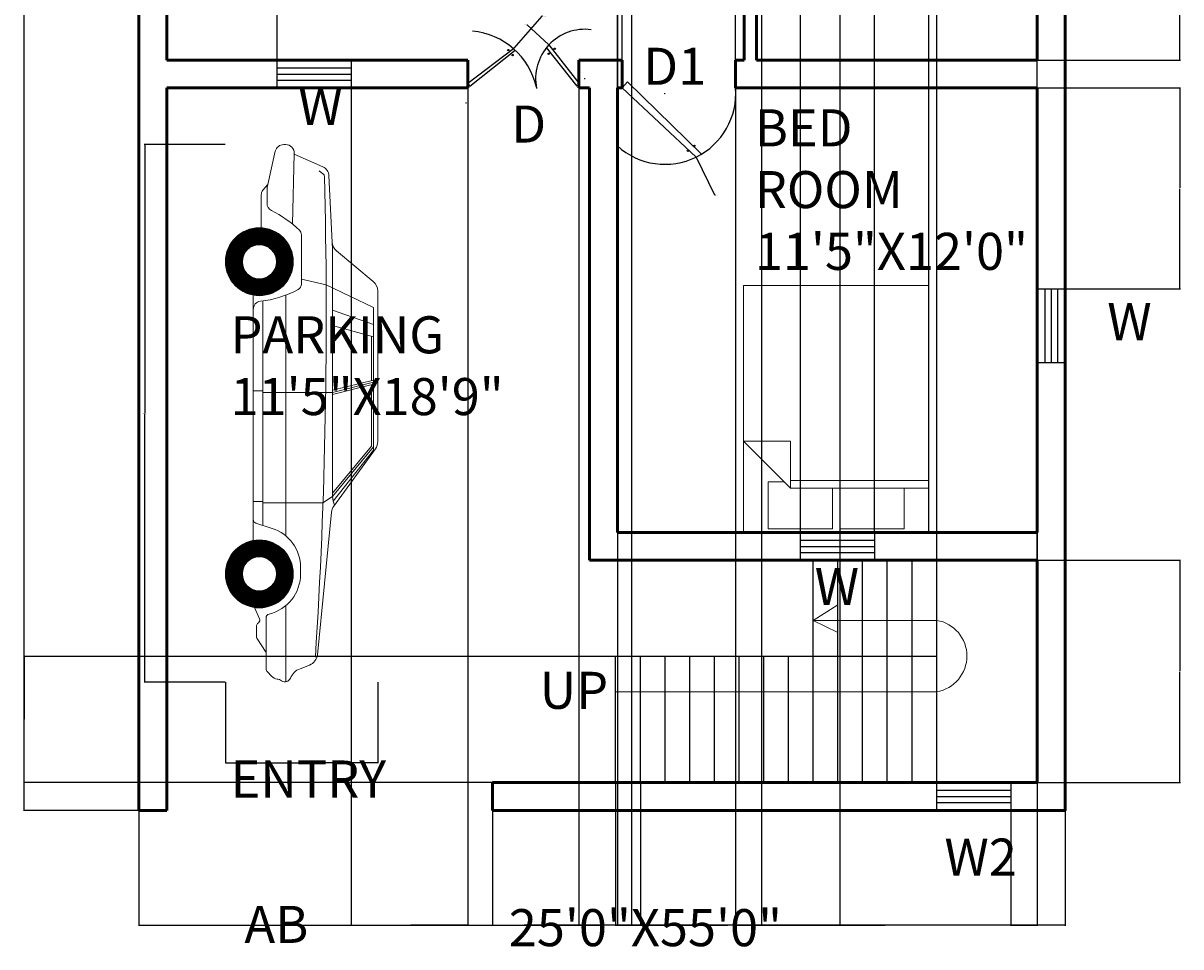
# Model space of a CAD drawing. Units: inches. Extents: x -15 to 361, y -684 to 58.
# Tile 1 of 3: x -15 to 360, y -684 to -385. Entities that reach past the tile are written whole.
import ezdxf

# ---------------------------------------------------------------- set-up
doc = ezdxf.new("R2010")
doc.units = ezdxf.units.IN
doc.header["$MEASUREMENT"] = 0
for name, color, linetype, lineweight in [('A-ANNO-DIMS', 2, 'Continuous', 18), ('A-ANNO-SYMB', 2, 'Continuous', 18), ('A-ANNO-TEXT', 7, 'Continuous', 18), ('A-AREA-IDEN', 7, 'Continuous', 25), ('A-DOOR', 3, 'Continuous', 25), ('A-EQPM-VEHC', 9, 'Continuous', 18), ('A-FLOR-STRS', 7, 'Continuous', 25), ('A-FURN', 8, 'Continuous', 18), ('A-GLAZ', 4, 'Continuous', 25), ('A-WALL', 7, 'Continuous', 50)]:
    doc.layers.add(name, color=color, linetype=linetype, lineweight=lineweight)
doc.styles.get("Standard").update_dxf_attribs({"font": 'arial.ttf'})
doc.dimstyles.get("Standard").update_dxf_attribs({"dimtxt": 0.18, "dimasz": 0.18, "dimexe": 0.18, "dimexo": 0.0625, "dimgap": 0.09, "dimtad": 0, "dimtih": 1, "dimtoh": 1, "dimdec": 4, "dimzin": 0, "dimdsep": 46, "dimtxsty": 'Standard', "dimcen": 0.09, "dimadec": 0, "dimazin": 0, "dimtfac": 1, "dimtdec": 4, "dimtofl": 0, "dimtmove": 0, "dimatfit": 3, "dimfxl": 1, "dimtolj": 1, "dimtzin": 0, "dimarcsym": 0})

# ---------------------------------------------------------------- blocks, each defined once
blk = doc.blocks.new('Bed - Queen')
for p, q in [((0, -80.00003), (0, 0)), ((0, 0), (59.99999, 0)), ((59.99999, 0), (59.99999, -80.00003)), ((7.99999, -1.2), (28.79998, -1.2)), ((7.99999, -14.4), (7.99999, -1.2)), ((28.79998, -1.2), (28.79998, -14.4)), ((31.19999, -1.2), (51.99999, -1.2)), ((31.19999, -14.4), (31.19999, -1.2)), ((51.99999, -1.2), (51.99999, -16.4)), ((0, -14.4), (44.8, -14.4)), ((59.99999, -29.6), (44.8, -14.4)), ((44.8, -14.4), (44.8, -29.6)), ((44.8, -16.8), (0, -16.8)), ((51.99999, -16.4), (46.79936, -16.4)), ((44.8, -29.6), (59.99999, -29.6)), ((59.99999, -80.00003), (0, -80.00003))]:
    blk.add_line(p, q)
blk = doc.blocks.new('Car - sedan  side')
for p, q in [((-77.81, 49.34), (-126.58, 49.34)), ((-139.53, 35.99), (-129.64, 47.91)), ((-128.57, 32.64), (-121.22, 48.02)), ((-74.7, 48.02), (-121.22, 48.02)), ((-120.32, 34.67), (-115.67, 48.02)), ((-115.4, 34.67), (-111.74, 48.02)), ((-97.55, 47.3), (-111.94, 47.3)), ((-94.41, 34.67), (-97.73, 48.02)), ((-93.72, 34.67), (-97.04, 48.02)), ((-93.03, 34.67), (-96.34, 48.02)), ((-76.26, 47.3), (-96.16, 47.3)), ((-61.08, 34.66), (-76.26, 47.3)), ((-60.02, 34.65), (-76.07, 48.02)), ((-56.87, 35.13), (-75.48, 48.59)), ((-58.54, 34.93), (-74.99, 48.02)), ((-140.23, 34.67), (-163.88, 33.56)), ((-62.28, 34.67), (-140.23, 34.67)), ((-93.72, 19.62), (-93.72, 34.67)), ((-62.28, 34.67), (-60.02, 34.65)), ((-60.02, 34.65), (-58.54, 34.93)), ((-57.97, 31.61), (-60.02, 34.65)), ((-57.21, 35.38), (-58.54, 34.93)), ((-54.93, 34.4), (-8.75, 29.8)), ((-170.93, 22.32), (-166.81, 31.56)), ((-164.57, 31.6), (-165.48, 30.35)), ((-130.39, 24.63), (-128.57, 32.64)), ((-57.97, 19.62), (-57.97, 31.61)), ((-4.21, 24.18), (-5.42, 27.27)), ((-128.78, 24.63), (-144.79, 24.63)), ((-36.97, 24.38), (-34.94, 24.38)), ((-174, 19.51), (-174, 18.91)), ((-148.26, 21.7), (-171.11, 22.33)), ((-47.2, 19.62), (-125.23, 19.62)), ((-93.72, 12.14), (-93.72, 19.62)), ((-57.97, 12.14), (-57.97, 19.62)), ((0, 19.62), (-24.7, 19.62)), ((-160.12, 13.48), (-171.81, 16.16)), ((-51.4, 9.89), (-49.69, 15.14)), ((-159.22, 12.14), (-161.08, 13.7)), ((-155.01, 13.48), (-160.12, 13.48)), ((-147.03, 11.6), (-157.73, 11.6)), ((-50.67, 12.14), (-123.32, 12.14)), ((-94.21, 9.03), (-94.21, 12.14)), ((-58.39, 9.03), (-58.39, 12.14)), ((-4.23, 13.19), (-20.72, 13.19)), ((-9.5, 13.19), (-14.1, 10.2)), ((-3.22, 13.59), (-1.77, 14.97)), ((-120.62, 9.03), (-125.23, 9.03)), ((-45.76, 9.03), (-120.62, 9.03)), ((-20.36, 11.06), (-24.06, 9.44)), ((-18.83, 10.42), (-19.11, 10.76)), ((-14.68, 10.03), (-18.01, 10.03))]:
    blk.add_line(p, q)
at = {"const_width": 5.49}
for points in [[(-127.8, 11, -1), (-144.3, 11, -1)], [(-26.69, 11, -1), (-43.19, 11, -1)]]:
    blk.add_lwpolyline(points, format="xyb", close=True, dxfattribs=at)
for centre, radius in [((-136.05, 11), 11), ((-34.94, 11), 11), ((-136.05, 11), 5.51), ((-34.94, 11), 5.51)]:
    blk.add_circle(centre, radius)
for centre, radius, start, end in [((-126.58, 45.38), 3.97, 90, 140.3029), ((-77.81, 45.38), 3.97, 54.135, 90), ((-142.58, 38.53), 3.97, 272.6827, 320.3029), ((-54.54, 38.35), 3.97, 234.135, 264.3123), ((-163.72, 30.18), 3.38, 92.6827, 155.9736), ((-163.62, 30.91), 1.17, 91.491, 143.9553), ((-118.51, -1702.12), 1734.79, 86.34698, 91.49105), ((-9.15, 25.82), 4, 21.3107, 84.3123), ((-118.09, -2.78), 38.85, 136.3964, 152.9097), ((-144.79, 22.64), 1.98, 90, 136.3964), ((-128.78, 22.64), 1.98, 28.1371, 90), ((-157.14, 7.48), 34.14, 6.5135, 28.1371), ((-36.97, 11), 13.38, 90, 161.9732), ((-34.94, 11), 13.38, 13.5864, 90), ((0.9, 26.18), 5.49, 201.3107, 247.7048), ((-171.18, 19.51), 2.82, 88.4193, 180), ((-171.18, 18.91), 2.82, 180, 257.0905), ((-1.92, 19.3), 1.94, 325.3744, 67.7048), ((-3.82, 17.12), 2.96, 313.7173, 352.3839), ((2.46, 16.28), 3.37, 145.3744, 172.3839), ((-157.73, 13.93), 2.32, 230.1291, 270), ((-155.01, 16.1), 2.62, 270, 332.9097), ((-120.62, 11.65), 2.62, 186.5135, 270), ((-20.72, 14.43), 1.24, 193.5864, 270), ((-4.23, 14.65), 1.46, 270, 313.7173), ((-52.58, 10.27), 1.24, 270, 341.9732), ((-19.93, 10.09), 1.06, 39.301, 113.7159), ((-18.01, 11.09), 1.06, 219.301, 270), ((-14.68, 11.09), 1.06, 270, 303.047)]:
    blk.add_arc(centre, radius, start, end)
blk = doc.blocks.new('WIN-24IN')
for p, q in [((0, 6.5), (24, 6.5)), ((0, 4.5), (24, 4.5)), ((0, 2.5), (24, 2.5))]:
    blk.add_line(p, q)
blk.add_lwpolyline([(0, 9), (24, 9), (24, 0), (0, 0)], close=True)
blk = doc.blocks.new('*D21')
at = {"layer": 'A-ANNO-DIMS', "color": 0, "lineweight": -2, "transparency": 16777216}
for p, q in [((50.87, -424.03), (24.63, -424.03)), ((24.81, -424.21), (24.81, -510.91)), ((24.81, -597.97), (24.81, -511.27)), ((50.87, -598.15), (24.63, -598.15))]:
    blk.add_line(p, q, dxfattribs=at)
at = {"layer": 'A-ANNO-DIMS', "color": 0, "transparency": 16777216}
for points in [[(24.78, -424.21), (24.84, -424.21), (24.81, -424.03)], [(24.78, -597.97), (24.84, -597.97), (24.81, -598.15)]]:
    blk.add_solid(points, dxfattribs=at)
at = {"layer": 'Defpoints', "color": 0, "transparency": 16777216}
for p in [(50.93, -424.03), (24.81, -598.15), (50.93, -598.15)]:
    blk.add_point(p, dxfattribs=at)
at = {"layer": 'A-ANNO-DIMS', "color": 0, "transparency": 16777216, "insert": (24.81, -511.09), "char_height": 0.18, "attachment_point": 5}
blk.add_mtext('\\A1;SEDAN 174', dxfattribs=at)
blk = doc.blocks.new('*D22')
at = {"layer": 'A-ANNO-DIMS', "color": 0, "lineweight": -2, "transparency": 16777216}
for p, q in [((50.93, -598.21), (50.93, -624.44)), ((100.28, -598.21), (100.28, -624.44)), ((51.11, -624.26), (75.38, -624.26)), ((100.1, -624.26), (75.83, -624.26))]:
    blk.add_line(p, q, dxfattribs=at)
at = {"layer": 'A-ANNO-DIMS', "color": 0, "transparency": 16777216}
for points in [[(51.11, -624.23), (51.11, -624.29), (50.93, -624.26)], [(100.1, -624.23), (100.1, -624.29), (100.28, -624.26)]]:
    blk.add_solid(points, dxfattribs=at)
at = {"layer": 'Defpoints', "color": 0, "transparency": 16777216}
for p in [(50.93, -598.15), (100.28, -598.15), (100.28, -624.26)]:
    blk.add_point(p, dxfattribs=at)
at = {"layer": 'A-ANNO-DIMS', "color": 0, "transparency": 16777216, "insert": (75.6, -624.26), "char_height": 0.18, "attachment_point": 5}
blk.add_mtext('\\A1;49', dxfattribs=at)
blk = doc.blocks.new('*D23')
at = {"layer": 'A-ANNO-DIMS', "color": 0, "lineweight": -2, "transparency": 16777216}
for p, q in [((22.93, -639.75), (22.93, -677.07)), ((322.93, -639.75), (322.93, -677.07)), ((23.11, -676.89), (172.64, -676.89)), ((322.75, -676.89), (173.22, -676.89))]:
    blk.add_line(p, q, dxfattribs=at)
at = {"layer": 'A-ANNO-DIMS', "color": 0, "transparency": 16777216}
for points in [[(23.11, -676.86), (23.11, -676.92), (22.93, -676.89)], [(322.75, -676.86), (322.75, -676.92), (322.93, -676.89)]]:
    blk.add_solid(points, dxfattribs=at)
at = {"layer": 'Defpoints', "color": 0, "transparency": 16777216}
for p in [(22.93, -639.69), (322.93, -639.69), (322.93, -676.89)]:
    blk.add_point(p, dxfattribs=at)
at = {"layer": 'A-ANNO-DIMS', "color": 0, "transparency": 16777216, "insert": (172.93, -676.89), "char_height": 0.18, "attachment_point": 5}
blk.add_mtext('\\A1;300', dxfattribs=at)
blk = doc.blocks.new('*D24')
at = {"layer": 'A-ANNO-DIMS', "color": 0, "lineweight": -2, "transparency": 16777216}
for p, q in [((22.87, 20.31), (-14.45, 20.31)), ((-14.27, 20.13), (-14.27, -309.51)), ((-14.27, -639.51), (-14.27, -309.87)), ((22.87, -639.69), (-14.45, -639.69))]:
    blk.add_line(p, q, dxfattribs=at)
at = {"layer": 'A-ANNO-DIMS', "color": 0, "transparency": 16777216}
for points in [[(-14.3, 20.13), (-14.24, 20.13), (-14.27, 20.31)], [(-14.3, -639.51), (-14.24, -639.51), (-14.27, -639.69)]]:
    blk.add_solid(points, dxfattribs=at)
at = {"layer": 'Defpoints', "color": 0, "transparency": 16777216}
for p in [(-14.27, 20.31), (22.93, 20.31), (22.93, -639.69)]:
    blk.add_point(p, dxfattribs=at)
at = {"layer": 'A-ANNO-DIMS', "color": 0, "transparency": 16777216, "insert": (-14.27, -309.69), "char_height": 0.18, "attachment_point": 5}
blk.add_mtext('\\A1;660', dxfattribs=at)
blk = doc.blocks.new('*D29')
at = {"layer": 'A-ANNO-DIMS', "color": 0, "lineweight": -2, "transparency": 16777216}
for p, q in [((313.99, -405.69), (360.31, -405.69)), ((360.13, -405.87), (360.13, -438.03)), ((360.13, -470.56), (360.13, -438.4)), ((313.99, -470.74), (360.31, -470.74))]:
    blk.add_line(p, q, dxfattribs=at)
at = {"layer": 'A-ANNO-DIMS', "color": 0, "transparency": 16777216}
for points in [[(360.1, -405.87), (360.16, -405.87), (360.13, -405.69)], [(360.1, -470.56), (360.16, -470.56), (360.13, -470.74)]]:
    blk.add_solid(points, dxfattribs=at)
at = {"layer": 'Defpoints', "color": 0, "transparency": 16777216}
for p in [(313.93, -405.69), (313.93, -470.74), (360.13, -470.74)]:
    blk.add_point(p, dxfattribs=at)
at = {"layer": 'A-ANNO-DIMS', "color": 0, "transparency": 16777216, "insert": (360.13, -438.22), "char_height": 0.18, "attachment_point": 5}
blk.add_mtext('\\A1;65.05', dxfattribs=at)
blk = doc.blocks.new('*D30')
at = {"layer": 'A-ANNO-DIMS', "color": 0, "lineweight": -2, "transparency": 16777216}
for p, q in [((305.35, -639.75), (305.35, -677.07)), ((322.93, -639.75), (322.93, -677.07)), ((305.53, -676.89), (313.68, -676.89)), ((322.75, -676.89), (314.6, -676.89))]:
    blk.add_line(p, q, dxfattribs=at)
at = {"layer": 'A-ANNO-DIMS', "color": 0, "transparency": 16777216}
for points in [[(305.53, -676.86), (305.53, -676.92), (305.35, -676.89)], [(322.75, -676.86), (322.75, -676.92), (322.93, -676.89)]]:
    blk.add_solid(points, dxfattribs=at)
at = {"layer": 'Defpoints', "color": 0, "transparency": 16777216}
for p in [(305.35, -639.69), (322.93, -639.69), (322.93, -676.89)]:
    blk.add_point(p, dxfattribs=at)
at = {"layer": 'A-ANNO-DIMS', "color": 0, "transparency": 16777216, "insert": (314.14, -676.89), "char_height": 0.18, "attachment_point": 5}
blk.add_mtext('\\A1;17.575', dxfattribs=at)
blk = doc.blocks.new('*D31')
at = {"layer": 'A-ANNO-DIMS', "color": 0, "lineweight": -2, "transparency": 16777216}
for p, q in [((177.93, -549.63), (177.93, 57.69)), ((178.11, 57.51), (207.18, 57.51)), ((237.04, 57.51), (207.97, 57.51)), ((237.22, -549.63), (237.22, 57.69))]:
    blk.add_line(p, q, dxfattribs=at)
at = {"layer": 'A-ANNO-DIMS', "color": 0, "transparency": 16777216}
for points in [[(178.11, 57.54), (178.11, 57.48), (177.93, 57.51)], [(237.04, 57.54), (237.04, 57.48), (237.22, 57.51)]]:
    blk.add_solid(points, dxfattribs=at)
at = {"layer": 'Defpoints', "color": 0, "transparency": 16777216}
for p in [(237.22, 57.51), (177.93, -549.69), (237.22, -549.69)]:
    blk.add_point(p, dxfattribs=at)
at = {"layer": 'A-ANNO-DIMS', "color": 0, "transparency": 16777216, "insert": (207.57, 57.51), "char_height": 0.18, "attachment_point": 5}
blk.add_mtext('\\A1;59.29', dxfattribs=at)
blk = doc.blocks.new('*D32')
at = {"layer": 'A-ANNO-DIMS', "color": 0, "lineweight": -2, "transparency": 16777216}
for p, q in [((31.93, -396.63), (31.93, 57.69)), ((32.11, 57.51), (49.42, 57.51)), ((67.52, 57.51), (50.21, 57.51)), ((67.7, -396.63), (67.7, 57.69))]:
    blk.add_line(p, q, dxfattribs=at)
at = {"layer": 'A-ANNO-DIMS', "color": 0, "transparency": 16777216}
for points in [[(32.11, 57.54), (32.11, 57.48), (31.93, 57.51)], [(67.52, 57.54), (67.52, 57.48), (67.7, 57.51)]]:
    blk.add_solid(points, dxfattribs=at)
at = {"layer": 'Defpoints', "color": 0, "transparency": 16777216}
for p in [(67.7, 57.51), (31.93, -396.69), (67.7, -396.69)]:
    blk.add_point(p, dxfattribs=at)
at = {"layer": 'A-ANNO-DIMS', "color": 0, "transparency": 16777216, "insert": (49.81, 57.51), "char_height": 0.18, "attachment_point": 5}
blk.add_mtext('\\A1;35.77', dxfattribs=at)
blk = doc.blocks.new('*D35')
at = {"layer": 'A-ANNO-DIMS', "color": 0, "lineweight": -2, "transparency": 16777216}
for p, q in [((137.49, -630.75), (137.49, -677.07)), ((177.35, -630.75), (177.35, -677.07)), ((137.67, -676.89), (157.03, -676.89)), ((177.17, -676.89), (157.82, -676.89))]:
    blk.add_line(p, q, dxfattribs=at)
at = {"layer": 'A-ANNO-DIMS', "color": 0, "transparency": 16777216}
for points in [[(137.67, -676.86), (137.67, -676.92), (137.49, -676.89)], [(177.17, -676.86), (177.17, -676.92), (177.35, -676.89)]]:
    blk.add_solid(points, dxfattribs=at)
at = {"layer": 'Defpoints', "color": 0, "transparency": 16777216}
for p in [(137.49, -630.69), (177.35, -630.69), (177.35, -676.89)]:
    blk.add_point(p, dxfattribs=at)
at = {"layer": 'A-ANNO-DIMS', "color": 0, "transparency": 16777216, "insert": (157.42, -676.89), "char_height": 0.18, "attachment_point": 5}
blk.add_mtext('\\A1;39.86', dxfattribs=at)
blk = doc.blocks.new('*D37')
at = {"layer": 'A-ANNO-DIMS', "color": 0, "lineweight": -2, "transparency": 16777216}
for p, q in [((182.53, -153.75), (182.53, -677.07)), ((224.64, -153.75), (224.64, -677.07)), ((182.71, -676.89), (203.21, -676.89)), ((224.46, -676.89), (203.97, -676.89))]:
    blk.add_line(p, q, dxfattribs=at)
at = {"layer": 'A-ANNO-DIMS', "color": 0, "transparency": 16777216}
for points in [[(182.71, -676.86), (182.71, -676.92), (182.53, -676.89)], [(224.46, -676.86), (224.46, -676.92), (224.64, -676.89)]]:
    blk.add_solid(points, dxfattribs=at)
at = {"layer": 'Defpoints', "color": 0, "transparency": 16777216}
for p in [(182.53, -153.69), (224.64, -153.69), (224.64, -676.89)]:
    blk.add_point(p, dxfattribs=at)
at = {"layer": 'A-ANNO-DIMS', "color": 0, "transparency": 16777216, "insert": (203.59, -676.89), "char_height": 0.18, "attachment_point": 5}
blk.add_mtext('\\A1;42.11', dxfattribs=at)
blk = doc.blocks.new('*D40')
at = {"layer": 'A-ANNO-DIMS', "color": 0, "lineweight": -2, "transparency": 16777216}
for p, q in [((91.7, -405.75), (91.7, -677.07)), ((129.45, -405.75), (129.45, -677.07)), ((91.88, -676.89), (110.18, -676.89)), ((129.27, -676.89), (110.97, -676.89))]:
    blk.add_line(p, q, dxfattribs=at)
at = {"layer": 'A-ANNO-DIMS', "color": 0, "transparency": 16777216}
for points in [[(91.88, -676.86), (91.88, -676.92), (91.7, -676.89)], [(129.27, -676.86), (129.27, -676.92), (129.45, -676.89)]]:
    blk.add_solid(points, dxfattribs=at)
at = {"layer": 'Defpoints', "color": 0, "transparency": 16777216}
for p in [(91.7, -405.69), (129.45, -405.69), (129.45, -676.89)]:
    blk.add_point(p, dxfattribs=at)
at = {"layer": 'A-ANNO-DIMS', "color": 0, "transparency": 16777216, "insert": (110.57, -676.89), "char_height": 0.18, "attachment_point": 5}
blk.add_mtext('\\A1;37.75', dxfattribs=at)
blk = doc.blocks.new('*D41')
at = {"layer": 'A-ANNO-DIMS', "color": 0, "lineweight": -2, "transparency": 16777216}
for p, q in [((129.45, -405.75), (129.45, -677.07)), ((165.45, -405.75), (165.45, -677.07)), ((129.63, -676.89), (147.23, -676.89)), ((165.27, -676.89), (147.67, -676.89))]:
    blk.add_line(p, q, dxfattribs=at)
at = {"layer": 'A-ANNO-DIMS', "color": 0, "transparency": 16777216}
for points in [[(129.63, -676.86), (129.63, -676.92), (129.45, -676.89)], [(165.27, -676.86), (165.27, -676.92), (165.45, -676.89)]]:
    blk.add_solid(points, dxfattribs=at)
at = {"layer": 'Defpoints', "color": 0, "transparency": 16777216}
for p in [(129.45, -405.69), (165.45, -405.69), (165.45, -676.89)]:
    blk.add_point(p, dxfattribs=at)
at = {"layer": 'A-ANNO-DIMS', "color": 0, "transparency": 16777216, "insert": (147.45, -676.89), "char_height": 0.18, "attachment_point": 5}
blk.add_mtext('\\A1;36', dxfattribs=at)
blk = doc.blocks.new('*D42')
at = {"layer": 'A-ANNO-DIMS', "color": 0, "lineweight": -2, "transparency": 16777216}
for p, q in [((179.42, -396.63), (179.42, 57.69)), ((179.6, 57.51), (197.42, 57.51)), ((216.02, 57.51), (198.21, 57.51)), ((216.2, -396.63), (216.2, 57.69))]:
    blk.add_line(p, q, dxfattribs=at)
at = {"layer": 'A-ANNO-DIMS', "color": 0, "transparency": 16777216}
for points in [[(179.6, 57.54), (179.6, 57.48), (179.42, 57.51)], [(216.02, 57.54), (216.02, 57.48), (216.2, 57.51)]]:
    blk.add_solid(points, dxfattribs=at)
at = {"layer": 'Defpoints', "color": 0, "transparency": 16777216}
for p in [(216.2, 57.51), (179.42, -396.69), (216.2, -396.69)]:
    blk.add_point(p, dxfattribs=at)
at = {"layer": 'A-ANNO-DIMS', "color": 0, "transparency": 16777216, "insert": (197.81, 57.51), "char_height": 0.18, "attachment_point": 5}
blk.add_mtext('\\A1;36.78', dxfattribs=at)
blk = doc.blocks.new('*D43')
at = {"layer": 'A-ANNO-DIMS', "color": 0, "lineweight": -2, "transparency": 16777216}
for p, q in [((313.99, -558.69), (360.31, -558.69)), ((360.13, -558.87), (360.13, -594.51)), ((360.13, -630.51), (360.13, -594.87)), ((313.99, -630.69), (360.31, -630.69))]:
    blk.add_line(p, q, dxfattribs=at)
at = {"layer": 'A-ANNO-DIMS', "color": 0, "transparency": 16777216}
for points in [[(360.1, -558.87), (360.16, -558.87), (360.13, -558.69)], [(360.1, -630.51), (360.16, -630.51), (360.13, -630.69)]]:
    blk.add_solid(points, dxfattribs=at)
at = {"layer": 'Defpoints', "color": 0, "transparency": 16777216}
for p in [(313.93, -558.69), (313.93, -630.69), (360.13, -630.69)]:
    blk.add_point(p, dxfattribs=at)
at = {"layer": 'A-ANNO-DIMS', "color": 0, "transparency": 16777216, "insert": (360.13, -594.69), "char_height": 0.18, "attachment_point": 5}
blk.add_mtext('\\A1;72', dxfattribs=at)
blk = doc.blocks.new('*D44')
at = {"layer": 'A-ANNO-DIMS', "color": 0, "lineweight": -2, "transparency": 16777216}
for p, q in [((281.35, -558.63), (281.35, 57.69)), ((281.53, 57.51), (297.18, 57.51)), ((313.75, 57.51), (298.1, 57.51)), ((313.93, -558.63), (313.93, 57.69))]:
    blk.add_line(p, q, dxfattribs=at)
at = {"layer": 'A-ANNO-DIMS', "color": 0, "transparency": 16777216}
for points in [[(281.53, 57.54), (281.53, 57.48), (281.35, 57.51)], [(313.75, 57.54), (313.75, 57.48), (313.93, 57.51)]]:
    blk.add_solid(points, dxfattribs=at)
at = {"layer": 'Defpoints', "color": 0, "transparency": 16777216}
for p in [(313.93, 57.51), (281.35, -558.69), (313.93, -558.69)]:
    blk.add_point(p, dxfattribs=at)
at = {"layer": 'A-ANNO-DIMS', "color": 0, "transparency": 16777216, "insert": (297.64, 57.51), "char_height": 0.18, "attachment_point": 5}
blk.add_mtext('\\A1;32.575', dxfattribs=at)
blk = doc.blocks.new('*D45')
at = {"layer": 'A-ANNO-DIMS', "color": 0, "lineweight": -2, "transparency": 16777216}
for p, q in [((177.35, -630.75), (177.35, -677.07)), ((185.35, -630.75), (185.35, -677.07)), ((177.53, -676.89), (181.2, -676.89)), ((185.17, -676.89), (181.5, -676.89))]:
    blk.add_line(p, q, dxfattribs=at)
at = {"layer": 'A-ANNO-DIMS', "color": 0, "transparency": 16777216}
for points in [[(177.53, -676.86), (177.53, -676.92), (177.35, -676.89)], [(185.17, -676.86), (185.17, -676.92), (185.35, -676.89)]]:
    blk.add_solid(points, dxfattribs=at)
at = {"layer": 'Defpoints', "color": 0, "transparency": 16777216}
for p in [(177.35, -630.69), (185.35, -630.69), (185.35, -676.89)]:
    blk.add_point(p, dxfattribs=at)
at = {"layer": 'A-ANNO-DIMS', "color": 0, "transparency": 16777216, "insert": (181.35, -676.89), "char_height": 0.18, "attachment_point": 5}
blk.add_mtext('\\A1;8', dxfattribs=at)
blk = doc.blocks.new('*D46')
at = {"layer": 'A-ANNO-DIMS', "color": 0, "lineweight": -2, "transparency": 16777216}
for p, q in [((177.29, -589.86), (-14.45, -589.86)), ((-14.27, -590.04), (-14.27, -610.09)), ((-14.27, -630.51), (-14.27, -610.46)), ((177.29, -630.69), (-14.45, -630.69))]:
    blk.add_line(p, q, dxfattribs=at)
at = {"layer": 'A-ANNO-DIMS', "color": 0, "transparency": 16777216}
for points in [[(-14.3, -590.04), (-14.24, -590.04), (-14.27, -589.86)], [(-14.3, -630.51), (-14.24, -630.51), (-14.27, -630.69)]]:
    blk.add_solid(points, dxfattribs=at)
at = {"layer": 'Defpoints', "color": 0, "transparency": 16777216}
for p in [(-14.27, -589.86), (177.35, -589.86), (177.35, -630.69)]:
    blk.add_point(p, dxfattribs=at)
at = {"layer": 'A-ANNO-DIMS', "color": 0, "transparency": 16777216, "insert": (-14.27, -610.28), "char_height": 0.18, "attachment_point": 5}
blk.add_mtext('\\A1;40.83', dxfattribs=at)
blk = doc.blocks.new('*D47')
at = {"layer": 'A-ANNO-DIMS', "color": 0, "lineweight": -2, "transparency": 16777216}
for p, q in [((216.2, -405.75), (216.2, -677.07)), ((313.93, -405.75), (313.93, -677.07)), ((216.38, -676.89), (264.67, -676.89)), ((313.75, -676.89), (265.46, -676.89))]:
    blk.add_line(p, q, dxfattribs=at)
at = {"layer": 'A-ANNO-DIMS', "color": 0, "transparency": 16777216}
for points in [[(216.38, -676.86), (216.38, -676.92), (216.2, -676.89)], [(313.75, -676.86), (313.75, -676.92), (313.93, -676.89)]]:
    blk.add_solid(points, dxfattribs=at)
at = {"layer": 'Defpoints', "color": 0, "transparency": 16777216}
for p in [(216.2, -405.69), (313.93, -405.69), (313.93, -676.89)]:
    blk.add_point(p, dxfattribs=at)
at = {"layer": 'A-ANNO-DIMS', "color": 0, "transparency": 16777216, "insert": (265.07, -676.89), "char_height": 0.18, "attachment_point": 5}
blk.add_mtext('\\A1;97.72', dxfattribs=at)
blk = doc.blocks.new('*D48')
at = {"layer": 'A-ANNO-DIMS', "color": 0, "lineweight": -2, "transparency": 16777216}
for p, q in [((222.99, -315.69), (360.31, -315.69)), ((360.13, -315.87), (360.13, -356.01)), ((360.13, -396.51), (360.13, -356.37)), ((222.99, -396.69), (360.31, -396.69))]:
    blk.add_line(p, q, dxfattribs=at)
at = {"layer": 'A-ANNO-DIMS', "color": 0, "transparency": 16777216}
for points in [[(360.1, -315.87), (360.16, -315.87), (360.13, -315.69)], [(360.1, -396.51), (360.16, -396.51), (360.13, -396.69)]]:
    blk.add_solid(points, dxfattribs=at)
at = {"layer": 'Defpoints', "color": 0, "transparency": 16777216}
for p in [(222.93, -315.69), (360.13, -315.69), (222.93, -396.69)]:
    blk.add_point(p, dxfattribs=at)
at = {"layer": 'A-ANNO-DIMS', "color": 0, "transparency": 16777216, "insert": (360.13, -356.19), "char_height": 0.18, "attachment_point": 5}
blk.add_mtext('\\A1;81', dxfattribs=at)
blk = doc.blocks.new('*D50')
at = {"layer": 'A-ANNO-DIMS', "color": 0, "lineweight": -2, "transparency": 16777216}
for p, q in [((177.93, -234.75), (177.93, -677.07)), ((249.93, -234.75), (249.93, -677.07)), ((178.11, -676.89), (213.71, -676.89)), ((249.75, -676.89), (214.15, -676.89))]:
    blk.add_line(p, q, dxfattribs=at)
at = {"layer": 'A-ANNO-DIMS', "color": 0, "transparency": 16777216}
for points in [[(178.11, -676.86), (178.11, -676.92), (177.93, -676.89)], [(249.75, -676.86), (249.75, -676.92), (249.93, -676.89)]]:
    blk.add_solid(points, dxfattribs=at)
at = {"layer": 'Defpoints', "color": 0, "transparency": 16777216}
for p in [(177.93, -234.69), (249.93, -234.69), (249.93, -676.89)]:
    blk.add_point(p, dxfattribs=at)
at = {"layer": 'A-ANNO-DIMS', "color": 0, "transparency": 16777216, "insert": (213.93, -676.89), "char_height": 0.18, "attachment_point": 5}
blk.add_mtext('\\A1;72', dxfattribs=at)
blk = doc.blocks.new('*D52')
at = {"layer": 'A-ANNO-DIMS', "color": 0, "lineweight": -2, "transparency": 16777216}
for p, q in [((261.22, -549.63), (261.22, 57.69)), ((261.4, 57.51), (269.54, 57.51)), ((278.6, 57.51), (270.45, 57.51)), ((278.78, -549.63), (278.78, 57.69))]:
    blk.add_line(p, q, dxfattribs=at)
at = {"layer": 'A-ANNO-DIMS', "color": 0, "transparency": 16777216}
for points in [[(261.4, 57.54), (261.4, 57.48), (261.22, 57.51)], [(278.6, 57.54), (278.6, 57.48), (278.78, 57.51)]]:
    blk.add_solid(points, dxfattribs=at)
at = {"layer": 'Defpoints', "color": 0, "transparency": 16777216}
for p in [(278.78, 57.51), (261.22, -549.69), (278.78, -549.69)]:
    blk.add_point(p, dxfattribs=at)
at = {"layer": 'A-ANNO-DIMS', "color": 0, "transparency": 16777216, "insert": (270, 57.51), "char_height": 0.18, "attachment_point": 5}
blk.add_mtext('\\A1;17.564', dxfattribs=at)
blk = doc.blocks.new('*D57')
at = {"layer": 'A-ANNO-DIMS', "color": 0, "lineweight": -2, "transparency": 16777216}
for p, q in [((193.23, -407.47), (193.41, -407.47)), ((193.32, -407.56), (193.32, -407.38)), ((209.51, -440.43), (203.52, -428.23)), ((209.69, -440.43), (209.51, -440.43))]:
    blk.add_line(p, q, dxfattribs=at)
at = {"layer": 'A-ANNO-DIMS', "color": 0, "transparency": 16777216}
blk.add_solid([(203.55, -428.22), (203.49, -428.25), (203.44, -428.07)], dxfattribs=at)
at = {"layer": 'Defpoints', "color": 0, "transparency": 16777216}
for p in [(193.32, -407.47), (203.44, -428.07)]:
    blk.add_point(p, dxfattribs=at)
at = {"layer": 'A-ANNO-DIMS', "color": 0, "transparency": 16777216, "insert": (210.17, -440.43), "char_height": 0.18, "attachment_point": 5}
blk.add_mtext('\\A1;R22.95', dxfattribs=at)
blk = doc.blocks.new('*D58')
at = {"layer": 'A-ANNO-DIMS', "color": 0, "lineweight": -2, "transparency": 16777216}
for p, q in [((153.48, -382.49), (144.4, -392.86)), ((153.66, -382.49), (153.48, -382.49)), ((128.87, -410.51), (129.05, -410.51)), ((128.96, -410.6), (128.96, -410.42))]:
    blk.add_line(p, q, dxfattribs=at)
at = {"layer": 'A-ANNO-DIMS', "color": 0, "transparency": 16777216}
blk.add_solid([(144.38, -392.84), (144.42, -392.88), (144.28, -393)], dxfattribs=at)
at = {"layer": 'Defpoints', "color": 0, "transparency": 16777216}
for p in [(144.28, -393), (128.96, -410.51)]:
    blk.add_point(p, dxfattribs=at)
at = {"layer": 'A-ANNO-DIMS', "color": 0, "transparency": 16777216, "insert": (154.21, -382.49), "char_height": 0.18, "attachment_point": 5}
blk.add_mtext('\\A1;R23.274', dxfattribs=at)
blk = doc.blocks.new('*D59')
at = {"layer": 'A-ANNO-DIMS', "color": 0, "lineweight": -2, "transparency": 16777216}
for p, q in [((148.53, -385.25), (148.71, -385.25)), ((148.71, -385.25), (155.58, -391.65)), ((167.29, -402.65), (167.47, -402.65)), ((167.38, -402.74), (167.38, -402.56))]:
    blk.add_line(p, q, dxfattribs=at)
at = {"layer": 'A-ANNO-DIMS', "color": 0, "transparency": 16777216}
blk.add_solid([(155.6, -391.63), (155.56, -391.67), (155.71, -391.77)], dxfattribs=at)
at = {"layer": 'Defpoints', "color": 0, "transparency": 16777216}
for p in [(155.71, -391.77), (167.38, -402.65)]:
    blk.add_point(p, dxfattribs=at)
at = {"layer": 'A-ANNO-DIMS', "color": 0, "transparency": 16777216, "insert": (148.05, -385.25), "char_height": 0.18, "attachment_point": 5}
blk.add_mtext('\\A1;R15.95', dxfattribs=at)

msp = doc.modelspace()

# ---------------------------------------------------------------- linework, layer by layer
at = {"layer": 'A-ANNO-SYMB'}
for p, q in [((249.3528, -573.1371), (241.3528, -578.1469)), ((241.3528, -578.1469), (281.3528, -578.1469)), ((241.3528, -578.1469), (249.3528, -582.0886)), ((281.3528, -601.2576), (177.3528, -601.2576))]:
    msp.add_line(p, q, dxfattribs=at)
msp.add_arc((279.4336, -589.7023), 11.7137, 279.430043, 80.569957, dxfattribs=at)
at = {"layer": 'A-DOOR'}
for p, q in [((144.2832, -392.9993), (129.451, -404.2941)), ((130.0676, -405.1039), (144.8257, -393.4891)), ((164.9235, -405.0802), (154.9933, -392.6022)), ((155.7137, -391.7745), (165.451, -404.1667)), ((129.451, -404.2941), (130.0676, -405.1039)), ((165.451, -404.1667), (164.9235, -405.0802)), ((179.4234, -405.6922), (181.2307, -403.7527)), ((181.2307, -403.7527), (205.1964, -427.1141)), ((203.4419, -428.073), (179.4234, -405.6922)), ((179.4234, -405.6922), (179.4234, -405.6922))]:
    msp.add_line(p, q, dxfattribs=at)
for centre in [(142.5761, -393.4388), (157.5984, -393.0128), (143.9503, -395.0481), (155.608, -394.6221), (200.7648, -426.0177), (202.8815, -424.4734)]:
    msp.add_circle(centre, 0.216, dxfattribs=at)
for centre, radius, start, end in [((128.958, -410.5149), 23.2736, 12.53599, 85.095507), ((167.3781, -402.6541), 15.9507, 82.507582, 191.480132), ((193.3239, -407.474), 22.9497, 227.866667, 4.452905)]:
    msp.add_arc(centre, radius, start, end, dxfattribs=at)
at = {"layer": 'A-FLOR-STRS'}
for p, q in [((241.3528, -630.6922), (241.3528, -558.6922)), ((249.3528, -630.6922), (249.3528, -558.6922)), ((257.3528, -630.6922), (257.3528, -558.6922)), ((265.3528, -630.6922), (265.3528, -558.6922)), ((273.3528, -630.6922), (273.3528, -558.6922)), ((281.3528, -630.6922), (281.3528, -558.6922)), ((177.3528, -630.6922), (177.3528, -589.8606)), ((281.3528, -589.8606), (177.3528, -589.8606)), ((185.3528, -630.6922), (185.3528, -589.8606)), ((193.3528, -630.6922), (193.3528, -589.8606)), ((201.3528, -630.6922), (201.3528, -589.8606)), ((209.3528, -630.6922), (209.3528, -589.8606)), ((217.3528, -630.6922), (217.3528, -589.8606)), ((225.3528, -630.6922), (225.3528, -589.8606)), ((233.3528, -630.6922), (233.3528, -589.8606))]:
    msp.add_line(p, q, dxfattribs=at)
at = {"layer": 'A-WALL'}
for p, q in [((31.9279, -396.6922), (31.9279, -234.6922)), ((313.9279, -234.6922), (313.9279, -396.6922)), ((218.9279, -315.6922), (218.9279, -396.6922)), ((222.9279, -315.6922), (222.9279, -396.6922)), ((31.9279, -396.6922), (129.451, -396.6922)), ((129.451, -396.6922), (129.451, -405.6922)), ((165.451, -396.6922), (165.451, -405.6922)), ((165.451, -396.6922), (179.4234, -396.6922)), ((179.4234, -396.6922), (179.4234, -405.6922)), ((216.2043, -396.6922), (216.2043, -405.6922)), ((216.2043, -396.6922), (218.9279, -396.6922)), ((222.9279, -396.6922), (313.9279, -396.6922)), ((31.9279, -630.6922), (31.9279, -405.6922)), ((31.9279, -405.6922), (129.451, -405.6922)), ((165.451, -405.6922), (168.9279, -405.6922)), ((168.9279, -558.6922), (168.9279, -405.6922)), ((177.9279, -549.6922), (177.9279, -405.6922)), ((177.9279, -405.6922), (179.4234, -405.6922)), ((216.2043, -405.6922), (313.9279, -405.6922)), ((313.9279, -405.6922), (313.9279, -549.6922)), ((177.9279, -549.6922), (313.9279, -549.6922)), ((168.9279, -558.6922), (313.9279, -558.6922)), ((313.9279, -558.6922), (313.9279, -630.6922)), ((31.9279, -630.6922), (31.9279, -639.6922)), ((313.9279, -630.6922), (137.4946, -630.6922)), ((137.4946, -630.6922), (137.4946, -639.6922))]:
    msp.add_line(p, q, dxfattribs=at)
msp.add_lwpolyline([(31.9279, -639.6922), (22.9279, -639.6922), (22.9279, 20.3078), (322.9279, 20.3078), (322.9279, -639.6922), (137.4946, -639.6922)], dxfattribs=at)

# ---------------------------------------------------------------- block references
at = {"layer": 'A-EQPM-VEHC', "rotation": 270}
msp.add_blockref('Car - sedan  side', (50.9318, -598.033), dxfattribs=at)
at = {"layer": 'A-FURN', "rotation": 180}
msp.add_blockref('Bed - Queen', (278.7809, -549.6922), dxfattribs=at)
at = {"layer": 'A-GLAZ'}
for p in [(67.6969, -405.692), (237.216, -558.692), (281.3524, -639.692)]:
    msp.add_blockref('WIN-24IN', p, dxfattribs=at)
at = {"layer": 'A-GLAZ', "rotation": 270.0000000000002}
msp.add_blockref('WIN-24IN', (313.9281, -470.7398), dxfattribs=at)

# ---------------------------------------------------------------- texts
at = {"layer": 'A-ANNO-TEXT', "char_height": 12, "attachment_point": 1}
for s, width, insert in [('D1', 17.014829, (186.3101, -392.6755)), ('W', 28.818045, (74.5345, -405.6922)), ('D', 13.546935, (143.5508, -411.3996)), ('W', 28.6293, (336.5998, -475.393)), ('W', 13.934232, (241.8299, -561.2105)), ('UP', 19.419795, (152.7497, -594.8081)), ('ENTRY', 67.268921, (52.6174, -623.5312)), ('W2', 31.561762, (283.8565, -648.8296)), ('AB', 66.281347, (57.0923, -670.6297)), ('25\'0"X55\'0"', 314.603004, (142.7316, -671.684))]:
    msp.add_mtext_dynamic_manual_height_columns(s, width=width, gutter_width=60, heights=[0], dxfattribs=dict(at, insert=insert))
at = {"layer": 'A-AREA-IDEN', "char_height": 12, "attachment_point": 1}
for s, width, insert in [('BED ROOM\\P11\'5"X12\'0"', 66.115361, (222.4138, -412.6171)), ('PARKING\\P11\'5"X18\'9"', 92.595692, (52.5864, -479.6554))]:
    msp.add_mtext_dynamic_manual_height_columns(s, width=width, gutter_width=60, heights=[0], dxfattribs=dict(at, insert=insert))

# ---------------------------------------------------------------- dimensions: what is measured, and where the dimension line sits
at = {"layer": 'A-ANNO-DIMS'}
for base, p1, p2, override, picture, middle in [((67.6973, 57.5078), (31.9279, -396.6922), (67.6973, -396.6922), {"dimdec": 2, "dimlfac": 1, "dimrnd": 0, "dimzin": 0, "dimdsep": 46, "dimlunit": 2}, '*D32', (49.8126, 57.5078)), ((237.2164, 57.5078), (177.9279, -549.6922), (237.2164, -549.6922), {"dimdec": 2, "dimlfac": 1, "dimrnd": 0, "dimzin": 0, "dimdsep": 46, "dimlunit": 2}, '*D31', (207.5721, 57.5078)), ((216.2043, 57.5078), (179.4234, -396.6922), (216.2043, -396.6922), {"dimdec": 2, "dimlfac": 1, "dimrnd": 0, "dimzin": 0, "dimdsep": 46, "dimlunit": 2}, '*D42', (197.8139, 57.5078)), ((278.78086, 57.50778), (261.21639, -549.69222), (278.78086, -549.69222), {"dimdec": 3, "dimlfac": 1, "dimrnd": 0, "dimzin": 0, "dimdsep": 46, "dimlunit": 2}, '*D52', (269.99863, 57.50778)), ((313.9279, 57.5078), (281.3528, -558.6922), (313.9279, -558.6922), {"dimdec": 3, "dimlfac": 1, "dimrnd": 0, "dimzin": 0, "dimdsep": 46, "dimlunit": 2}, '*D44', (297.6403, 57.5078)), ((224.6415, -676.8922), (182.5334, -153.6922), (224.6415, -153.6922), {"dimdec": 2, "dimlfac": 1, "dimrnd": 0, "dimzin": 0, "dimdsep": 46, "dimlunit": 2}, '*D37', (203.5874, -676.8922)), ((249.9279, -676.8922), (177.9279, -234.6922), (249.9279, -234.6922), {"dimdec": 0, "dimlfac": 1, "dimrnd": 0, "dimzin": 0, "dimdsep": 46, "dimlunit": 2}, '*D50', (213.9279, -676.8922)), ((129.451, -676.8922), (91.6973, -405.6922), (129.451, -405.6922), {"dimdec": 2, "dimlfac": 1, "dimrnd": 0, "dimzin": 0, "dimdsep": 46, "dimlunit": 2}, '*D40', (110.5741, -676.8922)), ((165.451, -676.8922), (129.451, -405.6922), (165.451, -405.6922), {"dimdec": 0, "dimlfac": 1, "dimrnd": 0, "dimzin": 0, "dimdsep": 46, "dimlunit": 2}, '*D41', (147.451, -676.8922)), ((313.9279, -676.8922), (216.2043, -405.6922), (313.9279, -405.6922), {"dimdec": 2, "dimlfac": 1, "dimrnd": 0, "dimzin": 0, "dimdsep": 46, "dimlunit": 2}, '*D47', (265.0661, -676.8922)), ((100.2767, -624.2639), (50.9318, -598.1468), (100.2767, -598.1468), {"dimdec": 0, "dimlfac": 1, "dimrnd": 0, "dimzin": 0, "dimdsep": 46, "dimlunit": 2}, '*D22', (75.6042, -624.2639)), ((177.3528, -676.8922), (137.4946, -630.6922), (177.3528, -630.6922), {"dimdec": 2, "dimlfac": 1, "dimrnd": 0, "dimzin": 0, "dimdsep": 46, "dimlunit": 2}, '*D35', (157.4237, -676.8922)), ((185.3528, -676.8922), (177.3528, -630.6922), (185.3528, -630.6922), {"dimdec": 0, "dimlfac": 1, "dimrnd": 0, "dimzin": 0, "dimdsep": 46, "dimlunit": 2}, '*D45', (181.3528, -676.8922)), ((322.9279, -676.8922), (22.9279, -639.6922), (322.9279, -639.6922), {"dimdec": 0, "dimlfac": 1, "dimrnd": 0, "dimzin": 0, "dimdsep": 46, "dimlunit": 2}, '*D23', (172.9279, -676.8922)), ((322.9279, -676.8922), (305.3528, -639.6922), (322.9279, -639.6922), {"dimdec": 3, "dimlfac": 1, "dimrnd": 0, "dimzin": 0, "dimdsep": 46, "dimlunit": 2}, '*D30', (314.1403, -676.8922))]:
    dim = msp.add_linear_dim(base=base, p1=p1, p2=p2, dimstyle='Standard', override=override, dxfattribs=at)
    dim.commit()
    dim.dimension.update_dxf_attribs({"geometry": picture, "text_midpoint": middle})
for base, p1, p2, override, picture, middle in [((-14.2721, 20.3078), (22.9279, -639.6922), (22.9279, 20.3078), {"dimdec": 0, "dimlfac": 1, "dimrnd": 0, "dimzin": 0, "dimdsep": 46, "dimlunit": 2}, '*D24', (-14.2721, -309.6922)), ((360.1279, -315.6922), (222.9279, -396.6922), (222.9279, -315.6922), {"dimdec": 0, "dimlfac": 1, "dimrnd": 0, "dimzin": 0, "dimdsep": 46, "dimlunit": 2}, '*D48', (360.1279, -356.1922)), ((360.1279, -470.7402), (313.9279, -405.6922), (313.9279, -470.7402), {"dimdec": 2, "dimlfac": 1, "dimrnd": 0, "dimzin": 0, "dimdsep": 46, "dimlunit": 2}, '*D29', (360.1279, -438.2162)), ((360.1279, -630.6922), (313.9279, -558.6922), (313.9279, -630.6922), {"dimdec": 0, "dimlfac": 1, "dimrnd": 0, "dimzin": 0, "dimdsep": 46, "dimlunit": 2}, '*D43', (360.1279, -594.6922)), ((-14.2721, -589.8606), (177.3528, -630.6922), (177.3528, -589.8606), {"dimdec": 2, "dimlfac": 1, "dimrnd": 0, "dimzin": 0, "dimdsep": 46, "dimlunit": 2}, '*D46', (-14.2721, -610.2764))]:
    dim = msp.add_linear_dim(base=base, p1=p1, p2=p2, angle=90, dimstyle='Standard', override=override, dxfattribs=at)
    dim.commit()
    dim.dimension.update_dxf_attribs({"geometry": picture, "text_midpoint": middle})
for center, mpoint, override, picture, middle in [((128.958, -410.5149), (144.283, -392.999), {"dimdec": 3, "dimlfac": 1, "dimrnd": 0, "dimzin": 0, "dimdsep": 46, "dimlunit": 2}, '*D58', (154.2073, -382.4895)), ((167.3781, -402.6541), (155.7136, -391.7746), {"dimdec": 2, "dimlfac": 1, "dimrnd": 0, "dimzin": 0, "dimdsep": 46, "dimlunit": 2}, '*D59', (148.0544, -385.2469)), ((193.3239, -407.474), (203.442, -428.0729), {"dimdec": 2, "dimlfac": 1, "dimrnd": 0, "dimzin": 0, "dimdsep": 46, "dimlunit": 2}, '*D57', (210.1733, -440.4323))]:
    dim = msp.add_radius_dim(center=center, mpoint=mpoint, dimstyle='Standard', override=override, dxfattribs=at)
    dim.commit()
    dim.dimension.update_dxf_attribs({"geometry": picture, "text_midpoint": middle, "dimtype": 164})
dim = msp.add_linear_dim(base=(24.8147, -598.1468), p1=(50.9318, -424.033), p2=(50.9318, -598.1468), angle=270, text='SEDAN <>', dimstyle='Standard', override={"dimdec": 0, "dimlfac": 1, "dimrnd": 0, "dimzin": 0, "dimdsep": 46, "dimlunit": 2}, dxfattribs=at)
dim.commit()
dim.dimension.update_dxf_attribs({"geometry": '*D21', "text_midpoint": (24.8147, -511.0899)})

doc.saveas('drawing.dxf')
